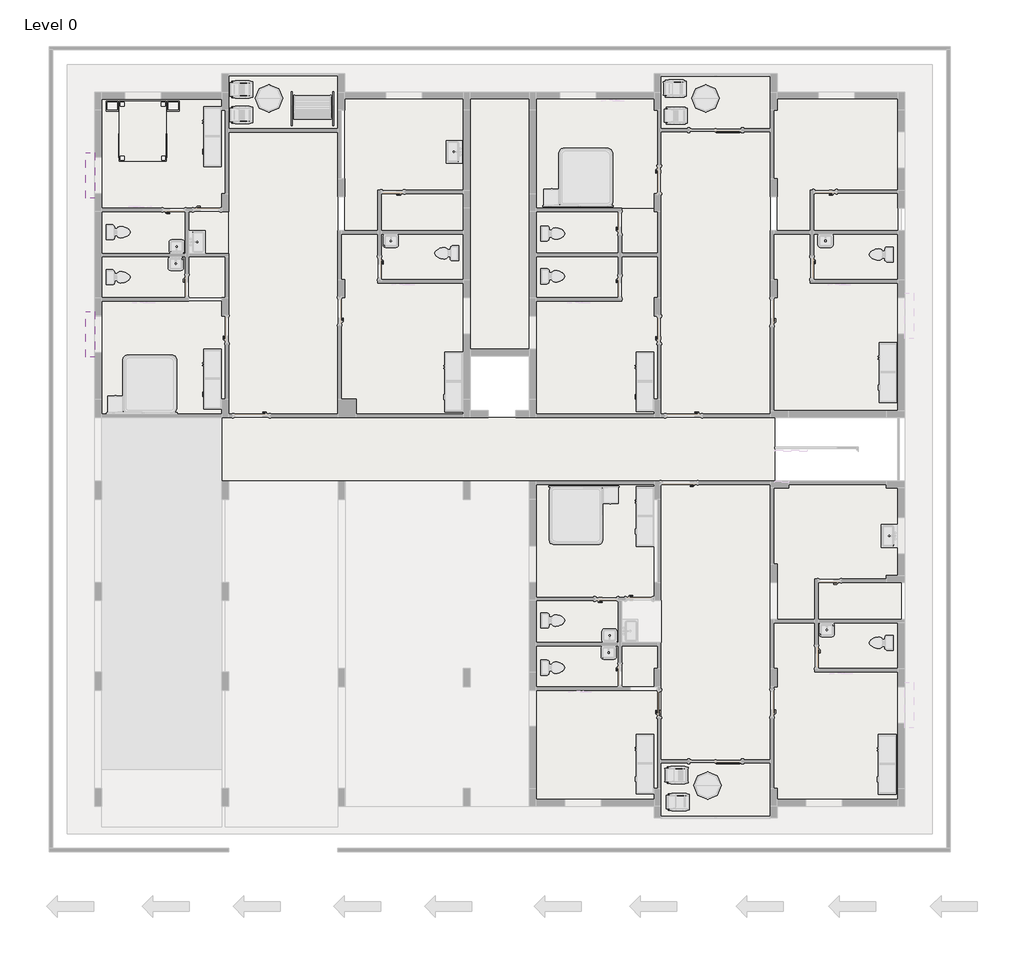
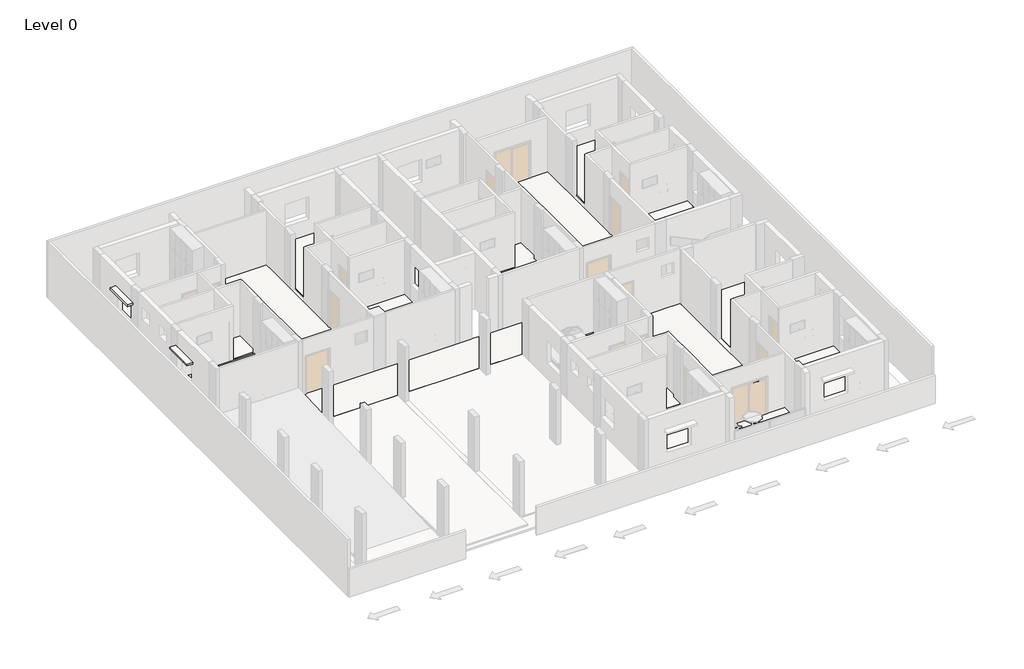
# One storey, part 4 of 6: 6 slabs.
"""IFC4 building model written with IfcOpenShell, lengths in millimetres."""

from ifc_helpers import new_model, si_unit, frame, origin, origin_with_axes, place, context, project, spatial, polyline, circle_curve, outline, extrude, element, save
from ifc_brep_helpers import plane_surface, cylinder_surface, revolved_surface, advanced_brep

model = new_model("IFC4")

# Units and contexts
model_context = context("Model", 3, world=origin())
ifc_project = project(units=[si_unit("LENGTHUNIT", "METRE", prefix="MILLI")], contexts=[model_context])

# Site, building, storey
site = spatial("IfcSite", under=ifc_project)
building = spatial("IfcBuilding", under=site)
storey = spatial("IfcBuildingStorey", under=building, Name="Level 0", Elevation=0.0)

# Slabs
placement = place(None, origin())
element("IfcSlab", 1, at=placement, inside=storey, context=model_context, shape_type="SweptSolid", body=[
    extrude(outline(polyline([(4028.5598466, -6653.8517861), (4028.5598466, -8050.8607795), (1285.3598461, -8050.8607795), (1285.3598461, -6653.8517861), (4028.5598466, -6653.8517861)])), frame((0.0, 0.0, -50.8), z_axis=(0.0, 0.0, 1.0), x_axis=(1.0, 0.0, 0.0)), (0.0, 0.0, 1.0), 50.8),
    extrude(outline(polyline([(4028.5598461, -8165.1517861), (4028.5598461, -9536.8048446), (1285.3598461, -9536.8048446), (1285.3598461, -8165.1517861), (4028.5598461, -8165.1517861)])), frame((0.0, 0.0, -50.8), z_axis=(0.0, 0.0, 1.0), x_axis=(1.0, 0.0, 0.0)), (0.0, 0.0, 1.0), 50.8),
    extrude(outline(polyline([(5343.0098461, -9536.7517862), (4142.8598461, -9536.7517862), (4142.8598461, -8165.1517861), (5343.0098461, -8165.1517861), (5343.0098461, -9536.7517862)])), frame((0.0, 0.0, -50.8), z_axis=(0.0, 0.0, 1.0), x_axis=(1.0, 0.0, 0.0)), (0.0, 0.0, 1.0), 50.8),
    extrude(outline(polyline([(10715.0567876, -7288.8517861), (10715.0567876, -6044.2517861), (13496.409846, -6044.2517861), (13496.409846, -7288.8517861), (10715.0567876, -7288.8517861)])), frame((0.0, 0.0, -50.8), z_axis=(0.0, 0.0, 1.0), x_axis=(1.0, 0.0, 0.0)), (0.0, 0.0, 1.0), 50.8),
    extrude(outline(polyline([(-5344.0401539, 10921.8022446), (-5344.0401539, 9143.8022446), (-9001.6401539, 9143.8022446), (-9001.6401539, 10921.8022446), (-5344.0401539, 10921.8022446)])), frame((0.0, 0.0, -50.8), z_axis=(0.0, 0.0, 1.0), x_axis=(1.0, 0.0, 0.0)), (0.0, 0.0, 1.0), 50.8),
    extrude(outline(polyline([(5462.3098461, -9651.0517861), (5462.3098461, -10565.4518735), (5343.0098461, -10565.4518735), (5343.0098461, -12927.6517861), (5228.6965978, -12927.6517861), (5228.6965978, -13308.6517861), (1285.3598461, -13308.6517861), (1285.3598461, -9651.0517861), (5462.3098461, -9651.0517861)])), frame((0.0, 0.0, -50.8), z_axis=(0.0, 0.0, 1.0), x_axis=(1.0, 0.0, 0.0)), (0.0, 0.0, 1.0), 50.8),
    extrude(outline(polyline([(5462.3098461, -6653.8517861), (5462.3098461, -8050.8607795), (4142.8598461, -8050.8607795), (4142.8598461, -6653.8517861), (5462.3098461, -6653.8517861)])), frame((0.0, 0.0, -50.8), z_axis=(0.0, 0.0, 1.0), x_axis=(1.0, 0.0, 0.0)), (0.0, 0.0, 1.0), 50.8),
    extrude(outline(polyline([(-9001.6401539, 6361.3562752), (-9001.6401539, 4965.5022446), (-10335.1401539, 4965.5022446), (-10335.1401539, 6361.3562752), (-9001.6401539, 6361.3562752)])), frame((0.0, 0.0, -50.8), z_axis=(0.0, 0.0, 1.0), x_axis=(1.0, 0.0, 0.0)), (0.0, 0.0, 1.0), 50.8),
])
element("IfcSlab", 2, ObjectType="4\"", at=placement, inside=storey, context=model_context, shape_type="SweptSolid", body=[
    extrude(outline(polyline([(-13783.1901539, 3022.4022446), (-13478.3901539, 3022.4022446), (-13478.3901539, 1498.4022446), (-13783.1901539, 1498.4022446), (-13783.1901539, 3022.4022446)])), frame((0.0, 0.0, 2108.2), z_axis=(0.0, 0.0, 1.0), x_axis=(1.0, 0.0, 0.0)), (0.0, 0.0, 1.0), 101.6),
])
element("IfcSlab", 3, ObjectType="4\"", at=placement, inside=storey, context=model_context, shape_type="SweptSolid", body=[
    extrude(outline(polyline([(-13783.190154, 8342.5562752), (-13478.3901539, 8342.5562752), (-13478.3901539, 6818.5562752), (-13783.190154, 6818.5562752), (-13783.190154, 8342.5562752)])), frame((0.0, 0.0, 2108.2), z_axis=(0.0, 0.0, 1.0), x_axis=(1.0, 0.0, 0.0)), (0.0, 0.0, 1.0), 101.6),
])
element("IfcSlab", 4, ObjectType="Tile", at=placement, inside=storey, context=model_context, shape_type="AdvancedBrep", body=[
    advanced_brep(
    [(-9230.2401539, 10133.2562752, 0.0), (-9230.2401539, 9752.2562752, 0.0), (-9115.9401539, 9752.2562752, 0.0), (-9115.9401539, 6972.1022446, 0.0), (-9230.2401539, 6972.1022446, 0.0), (-9230.2401539, 6476.8022446, 0.0), (-13249.7901539, 6476.8022446, 0.0), (-13249.7901539, 10133.2562752, 0.0), (-12669.0887417, 8172.6340818, 0.0), (-12666.8305798, 8172.6340818, 0.0), (-12666.8305798, 8969.1064638, 0.0), (-12669.0887417, 8969.1064638, 0.0), (-12689.9697227, 10058.1316218, 0.0), (-13099.9697227, 10058.1316218, 0.0), (-13099.9697227, 9728.1316218, 0.0), (-12689.9697227, 9728.1316218, 0.0), (-10645.1697227, 10058.1316218, 0.0), (-11055.1697227, 10058.1316218, 0.0), (-11055.1697227, 9728.1316218, 0.0), (-10645.1697227, 9728.1316218, 0.0), (-12459.9697227, 8051.5316218, 0.0), (-12459.9697227, 8251.5316218, 0.0), (-12659.9697227, 8251.5316218, 0.0), (-12659.9697227, 8051.5316218, 0.0), (-11285.1697227, 8051.5316218, 0.0), (-11085.1697227, 8051.5316218, 0.0), (-11085.1697227, 8251.5316218, 0.0), (-11285.1697227, 8251.5316218, 0.0), (-11285.1697227, 10058.1316218, 0.0), (-11285.1697227, 9858.1316218, 0.0), (-11085.1697227, 9858.1316218, 0.0), (-11085.1697227, 10058.1316218, 0.0), (-12459.9697227, 10058.1316218, 0.0), (-12659.9697227, 10058.1316218, 0.0), (-12659.9697227, 9858.1316218, 0.0), (-12459.9697227, 9858.1316218, 0.0), (-9230.2401539, 9752.2562752, 76.2), (-9230.2401539, 10133.2562752, 76.2), (-13249.7901539, 10133.2562752, 76.2), (-13249.7901539, 6476.8022446, 76.2), (-9230.2401539, 6476.8022446, 76.2), (-9230.2401539, 6972.1022446, 76.2), (-9115.9401539, 6972.1022446, 76.2), (-9115.9401539, 9752.2562752, 76.2), (-12659.9697227, 10058.1316218, 76.2), (-11085.1697227, 10058.1316218, 76.2), (-11085.1697227, 8051.5316218, 76.2), (-12659.9697227, 8051.5316218, 76.2), (-10645.1697227, 9728.1316218, 76.2), (-11055.1697227, 9728.1316218, 76.2), (-11055.1697227, 10058.1316218, 76.2), (-10645.1697227, 10058.1316218, 76.2), (-12689.9697227, 9728.1316218, 76.2), (-13099.9697227, 9728.1316218, 76.2), (-13099.9697227, 10058.1316218, 76.2), (-12689.9697227, 10058.1316218, 76.2), (-12668.2662368, 8172.6340818, 76.2), (-12669.2815845, 8172.6340818, 76.2), (-12669.2815845, 8969.1064638, 76.2), (-12668.2662368, 8969.1064638, 76.2), (-11068.8512642, 8172.6340818, 76.2), (-11069.8590146, 8172.6340818, 76.2), (-11069.8590146, 8969.1064638, 76.2), (-11068.8512642, 8969.1064638, 76.2), (-11085.1697227, 8051.5316218, 60.0), (-11085.1697227, 10058.1316218, 60.0), (-12659.9697227, 10058.1316218, 60.0), (-12659.9697227, 8051.5316218, 60.0), (-12619.9697227, 10018.1316218, 60.0), (-12499.9697227, 10018.1316218, 60.0), (-12499.9697227, 9898.1316218, 60.0), (-12619.9697227, 9898.1316218, 60.0), (-11249.1033441, 10018.1316218, 60.0), (-11125.1697227, 10018.1316218, 60.0), (-11125.1697227, 9898.1316218, 60.0), (-11249.1033441, 9898.1316218, 60.0), (-12619.9697227, 8211.5316218, 60.0), (-12499.9697227, 8211.5316218, 60.0), (-12499.9697227, 8091.5316218, 60.0), (-12619.9697227, 8091.5316218, 60.0), (-11245.1697227, 8211.5316218, 60.0), (-11125.1697227, 8211.5316218, 60.0), (-11125.1697227, 8091.5316218, 60.0), (-11245.1697227, 8091.5316218, 60.0), (-10685.1697227, 10018.1316218, 50.0), (-10685.1697227, 10018.1316218, 60.0), (-11015.1697227, 10018.1316218, 60.0), (-11015.1697227, 10018.1316218, 50.0), (-11015.1697227, 9768.1316218, 60.0), (-11015.1697227, 9768.1316218, 50.0), (-10685.1697227, 9768.1316218, 60.0), (-10685.1697227, 9768.1316218, 50.0), (-12729.9697227, 10018.1316218, 50.0), (-12729.9697227, 10018.1316218, 60.0), (-13059.9697227, 10018.1316218, 60.0), (-13059.9697227, 10018.1316218, 50.0), (-13059.9697227, 9768.1316218, 60.0), (-13059.9697227, 9768.1316218, 50.0), (-12729.9697227, 9768.1316218, 60.0), (-12729.9697227, 9768.1316218, 50.0), (-11055.1697227, 10058.1316218, 60.0), (-11055.1697227, 9728.1316218, 60.0), (-10645.1697227, 9728.1316218, 60.0), (-10645.1697227, 10058.1316218, 60.0), (-13099.9697227, 10058.1316218, 60.0), (-13099.9697227, 9728.1316218, 60.0), (-12689.9697227, 9728.1316218, 60.0), (-12689.9697227, 10058.1316218, 60.0), (-12499.9697227, 10018.1316218, 50.0), (-12619.9697227, 10018.1316218, 50.0), (-12619.9697227, 9898.1316218, 50.0), (-12499.9697227, 9898.1316218, 50.0), (-11125.1697227, 10018.1316218, 50.0), (-11249.1033441, 10018.1316218, 50.0), (-11249.1033441, 9898.1316218, 50.0), (-11125.1697227, 9898.1316218, 50.0), (-12499.9697227, 8211.5316218, 50.0), (-12619.9697227, 8211.5316218, 50.0), (-12619.9697227, 8091.5316218, 50.0), (-12499.9697227, 8091.5316218, 50.0), (-11125.1697227, 8211.5316218, 50.0), (-11245.1697227, 8211.5316218, 50.0), (-11245.1697227, 8091.5316218, 50.0), (-11125.1697227, 8091.5316218, 50.0), (-11065.9668196, 8172.6340818, 0.0), (-11080.438493, 8172.6340818, 25.8475978), (-11079.4802179, 8172.6340818, 25.5617504), (-11065.1424088, 8172.6340818, 0.8244107), (-12680.5715859, 8172.6340818, 27.6877586), (-12679.6113712, 8172.6340818, 27.4084957), (-12679.6113712, 8969.1064638, 27.4084957), (-12680.5715859, 8969.1064638, 27.6877586), (-11065.1424088, 8969.1064638, 0.8244107), (-11079.4802179, 8969.1064638, 25.5617504), (-11080.438493, 8969.1064638, 25.8475978), (-11065.9668196, 8969.1064638, 0.0), (-13099.9697227, 10058.1316218, 50.0), (-12689.9697227, 10058.1316218, 50.0), (-12689.9697227, 9728.1316218, 50.0), (-13099.9697227, 9728.1316218, 50.0), (-11055.1697227, 10058.1316218, 50.0), (-10645.1697227, 10058.1316218, 50.0), (-10645.1697227, 9728.1316218, 50.0), (-11055.1697227, 9728.1316218, 50.0), (-12459.9697227, 8251.5316218, 50.0), (-12459.9697227, 8051.5316218, 50.0), (-12659.9697227, 8051.5316218, 50.0), (-12659.9697227, 8251.5316218, 50.0), (-11085.1697227, 8051.5316218, 50.0), (-11285.1697227, 8051.5316218, 50.0), (-11285.1697227, 8251.5316218, 50.0), (-11085.1697227, 8251.5316218, 50.0), (-11285.1697227, 9858.1316218, 50.0), (-11285.1697227, 10058.1316218, 50.0), (-11085.1697227, 10058.1316218, 50.0), (-11085.1697227, 9858.1316218, 50.0), (-12659.9697227, 10058.1316218, 50.0), (-12459.9697227, 10058.1316218, 50.0), (-12459.9697227, 9858.1316218, 50.0), (-12659.9697227, 9858.1316218, 50.0)],
    [
        (0, 1),
        (1, 2),
        (2, 3),
        (3, 4),
        (4, 5),
        (5, 6),
        (6, 7),
        (7, 0),
        (8, 9),
        (9, 10),
        (10, 11),
        (11, 8),
        (12, 13),
        (13, 14),
        (14, 15),
        (15, 12),
        (16, 17),
        (17, 18),
        (18, 19),
        (19, 16),
        (20, 21),
        (21, 22),
        (22, 23),
        (23, 20),
        (24, 25),
        (25, 26),
        (26, 27),
        (27, 24),
        (28, 29),
        (29, 30),
        (30, 31),
        (31, 28),
        (32, 33),
        (33, 34),
        (34, 35),
        (35, 32),
        (36, 37),
        (37, 38),
        (38, 39),
        (39, 40),
        (40, 41),
        (41, 42),
        (42, 43),
        (43, 36),
        (44, 45),
        (45, 46),
        (46, 47),
        (47, 44),
        (48, 49),
        (49, 50),
        (50, 51),
        (51, 48),
        (52, 53),
        (53, 54),
        (54, 55),
        (55, 52),
        (56, 57),
        (57, 58),
        (58, 59),
        (59, 56),
        (60, 61),
        (61, 62),
        (62, 63),
        (63, 60),
        (0, 37),
        (36, 1),
        (43, 2),
        (42, 3),
        (41, 4),
        (40, 5),
        (39, 6),
        (38, 7),
        (64, 65),
        (65, 66),
        (66, 67),
        (67, 64),
        (68, 69),
        (69, 70),
        (70, 71),
        (71, 68),
        (72, 73),
        (73, 74),
        (74, 75),
        (75, 72),
        (76, 77),
        (77, 78),
        (78, 79),
        (79, 76),
        (80, 81),
        (81, 82),
        (82, 83),
        (83, 80),
        (65, 45),
        (44, 66),
        (47, 67),
        (46, 64),
        (84, 85),
        (85, 86),
        (86, 87),
        (87, 84),
        (86, 88),
        (88, 89),
        (89, 87),
        (88, 90),
        (90, 91),
        (91, 89),
        (84, 91),
        (90, 85),
        (92, 93),
        (93, 94),
        (94, 95),
        (95, 92),
        (94, 96),
        (96, 97),
        (97, 95),
        (96, 98),
        (98, 99),
        (99, 97),
        (92, 99),
        (98, 93),
        (100, 101),
        (101, 102),
        (102, 103),
        (103, 100),
        (104, 105),
        (105, 106),
        (106, 107),
        (107, 104),
        (101, 49),
        (48, 102),
        (51, 103),
        (50, 100),
        (105, 53),
        (52, 106),
        (55, 107),
        (54, 104),
        (108, 69),
        (68, 109),
        (109, 108),
        (71, 110),
        (110, 109),
        (70, 111),
        (111, 110),
        (108, 111),
        (112, 73),
        (72, 113),
        (113, 112),
        (75, 114),
        (114, 113),
        (74, 115),
        (115, 114),
        (112, 115),
        (116, 77),
        (76, 117),
        (117, 116),
        (79, 118),
        (118, 117),
        (78, 119),
        (119, 118),
        (116, 119),
        (120, 81),
        (80, 121),
        (121, 120),
        (83, 122),
        (122, 121),
        (82, 123),
        (123, 122),
        (120, 123),
        (124, 125, circle_curve(frame((-11060.6581831, 8172.6340818, 19.947257), z_axis=(0.0, 1.0, 0.0), x_axis=(1.0, 0.0, 0.0)), 20.6415766)),
        (125, 61, circle_curve(frame((-11378.5350117, 8172.6340818, 114.7678954), z_axis=(0.0, -1.0, 0.0), x_axis=(1.0, 0.0, 0.0)), 311.0761221)),
        (60, 126, circle_curve(frame((-11378.5350117, 8172.6340818, 114.7678954), z_axis=(0.0, 1.0, 0.0), x_axis=(1.0, 0.0, 0.0)), 312.0761221)),
        (126, 127, circle_curve(frame((-11060.6581831, 8172.6340818, 19.947257), z_axis=(0.0, -1.0, 0.0), x_axis=(1.0, 0.0, 0.0)), 19.6415766)),
        (127, 124),
        (8, 128, circle_curve(frame((-12657.5756771, 8172.6340818, 20.9997703), z_axis=(0.0, 1.0, 0.0), x_axis=(1.0, 0.0, 0.0)), 23.9487162)),
        (128, 57, circle_curve(frame((-13120.6038463, 8172.6340818, 155.6640283), z_axis=(0.0, -1.0, 0.0), x_axis=(1.0, 0.0, 0.0)), 458.2644606)),
        (56, 129, circle_curve(frame((-13120.6038463, 8172.6340818, 155.6640283), z_axis=(0.0, 1.0, 0.0), x_axis=(1.0, 0.0, 0.0)), 459.2644606)),
        (129, 9, circle_curve(frame((-12657.5756771, 8172.6340818, 20.9997703), z_axis=(0.0, -1.0, 0.0), x_axis=(1.0, 0.0, 0.0)), 22.9487162)),
        (10, 130, circle_curve(frame((-12657.5756771, 8969.1064638, 20.9997703), z_axis=(0.0, 1.0, 0.0), x_axis=(1.0, 0.0, 0.0)), 22.9487162)),
        (130, 59, circle_curve(frame((-13120.6038463, 8969.1064638, 155.6640283), z_axis=(0.0, -1.0, 0.0), x_axis=(1.0, 0.0, 0.0)), 459.2644606)),
        (58, 131, circle_curve(frame((-13120.6038463, 8969.1064638, 155.6640283), z_axis=(0.0, 1.0, 0.0), x_axis=(1.0, 0.0, 0.0)), 458.2644606)),
        (131, 11, circle_curve(frame((-12657.5756771, 8969.1064638, 20.9997703), z_axis=(0.0, -1.0, 0.0), x_axis=(1.0, 0.0, 0.0)), 23.9487162)),
        (132, 133, circle_curve(frame((-11060.6581831, 8969.1064638, 19.947257), z_axis=(0.0, 1.0, 0.0), x_axis=(1.0, 0.0, 0.0)), 19.6415766)),
        (133, 63, circle_curve(frame((-11378.5350117, 8969.1064638, 114.7678954), z_axis=(0.0, -1.0, 0.0), x_axis=(1.0, 0.0, 0.0)), 312.0761221)),
        (62, 134, circle_curve(frame((-11378.5350117, 8969.1064638, 114.7678954), z_axis=(0.0, 1.0, 0.0), x_axis=(1.0, 0.0, 0.0)), 311.0761221)),
        (134, 135, circle_curve(frame((-11060.6581831, 8969.1064638, 19.947257), z_axis=(0.0, -1.0, 0.0), x_axis=(1.0, 0.0, 0.0)), 20.6415766)),
        (135, 132),
        (125, 134),
        (133, 126),
        (128, 131),
        (130, 129),
        (136, 137),
        (137, 138),
        (138, 139),
        (139, 136),
        (140, 141),
        (141, 142),
        (142, 143),
        (143, 140),
        (136, 13),
        (12, 137),
        (139, 14),
        (138, 15),
        (140, 17),
        (16, 141),
        (143, 18),
        (142, 19),
        (144, 145),
        (145, 146),
        (146, 147),
        (147, 144),
        (148, 149),
        (149, 150),
        (150, 151),
        (151, 148),
        (152, 153),
        (153, 154),
        (154, 155),
        (155, 152),
        (156, 157),
        (157, 158),
        (158, 159),
        (159, 156),
        (144, 21),
        (20, 145),
        (147, 22),
        (146, 23),
        (148, 25),
        (24, 149),
        (151, 26),
        (150, 27),
        (152, 29),
        (28, 153),
        (155, 30),
        (154, 31),
        (156, 33),
        (32, 157),
        (159, 34),
        (158, 35),
        (124, 135),
        (127, 132),
    ],
    [
        plane_surface(frame((-9230.2401539, 10361.8562752, 0.0), z_axis=(0.0, 0.0, -1.0), x_axis=(0.0, -1.0, 0.0))),
        plane_surface(frame((-9230.2401539, 10361.8562752, 76.2), z_axis=(0.0, 0.0, 1.0), x_axis=(0.0, 1.0, 0.0))),
        plane_surface(frame((-9230.2401539, 10133.2562752, 0.0), z_axis=(1.0, 0.0, 0.0), x_axis=(0.0, 0.0, 1.0))),
        plane_surface(frame((-9230.2401539, 9752.2562752, 0.0), z_axis=(0.0, 1.0, 0.0), x_axis=(0.0, 0.0, 1.0))),
        plane_surface(frame((-9115.9401539, 9752.2562752, 0.0), z_axis=(1.0, 0.0, 0.0), x_axis=(0.0, 0.0, 1.0))),
        plane_surface(frame((-9115.9401539, 6972.1022446, 0.0), z_axis=(0.0, -1.0, 0.0), x_axis=(0.0, 0.0, 1.0))),
        plane_surface(frame((-9230.2401539, 6972.1022446, 0.0), z_axis=(1.0, 0.0, 0.0), x_axis=(0.0, 0.0, 1.0))),
        plane_surface(frame((-9230.2401539, 6476.8022446, 0.0), z_axis=(0.0, -1.0, 0.0), x_axis=(0.0, 0.0, 1.0))),
        plane_surface(frame((-13249.7901539, 6476.8022446, 0.0), z_axis=(-1.0, 0.0, 0.0), x_axis=(0.0, 0.0, 1.0))),
        plane_surface(frame((-13249.7901539, 10133.2562752, 0.0), z_axis=(0.0, 1.0, 0.0), x_axis=(0.0, 0.0, 1.0))),
        plane_surface(frame((-12659.9697227, 10058.1316218, 60.0), z_axis=(0.0, 0.0, 1.0), x_axis=(1.0, 0.0, 0.0))),
        plane_surface(frame((-11085.1697227, 10058.1316218, 286.5360466), z_axis=(0.0, -1.0, 0.0), x_axis=(0.0, 0.0, -1.0))),
        plane_surface(frame((-12659.9697227, 10058.1316218, 286.5360466), z_axis=(1.0, 0.0, 0.0), x_axis=(0.0, 0.0, -1.0))),
        plane_surface(frame((-12659.9697227, 8051.5316218, 286.5360466), z_axis=(0.0, 1.0, 0.0), x_axis=(0.0, 0.0, -1.0))),
        plane_surface(frame((-11085.1697227, 8051.5316218, 286.5360466), z_axis=(-1.0, 0.0, 0.0), x_axis=(0.0, 0.0, -1.0))),
        plane_surface(frame((-10685.1697227, 10018.1316218, 60.0), z_axis=(0.0, -1.0, 0.0), x_axis=(0.0, 0.0, -1.0))),
        plane_surface(frame((-11015.1697227, 10018.1316218, 60.0), z_axis=(1.0, 0.0, 0.0), x_axis=(0.0, 0.0, -1.0))),
        plane_surface(frame((-11015.1697227, 9768.1316218, 60.0), z_axis=(0.0, 1.0, 0.0), x_axis=(0.0, 0.0, -1.0))),
        plane_surface(frame((-10685.1697227, 9768.1316218, 60.0), z_axis=(-1.0, 0.0, 0.0), x_axis=(0.0, 0.0, -1.0))),
        plane_surface(frame((-12729.9697227, 10018.1316218, 60.0), z_axis=(0.0, -1.0, 0.0), x_axis=(0.0, 0.0, -1.0))),
        plane_surface(frame((-13059.9697227, 10018.1316218, 60.0), z_axis=(1.0, 0.0, 0.0), x_axis=(0.0, 0.0, -1.0))),
        plane_surface(frame((-13059.9697227, 9768.1316218, 60.0), z_axis=(0.0, 1.0, 0.0), x_axis=(0.0, 0.0, -1.0))),
        plane_surface(frame((-12729.9697227, 9768.1316218, 60.0), z_axis=(-1.0, 0.0, 0.0), x_axis=(0.0, 0.0, -1.0))),
        plane_surface(frame((-10645.1697227, 9728.1316218, 60.0), z_axis=(0.0, 0.0, 1.0), x_axis=(-1.0, 0.0, 0.0))),
        plane_surface(frame((-11055.1697227, 9728.1316218, 350.5398437), z_axis=(0.0, 1.0, 0.0), x_axis=(0.0, 0.0, -1.0))),
        plane_surface(frame((-10645.1697227, 9728.1316218, 350.5398437), z_axis=(-1.0, 0.0, 0.0), x_axis=(0.0, 0.0, -1.0))),
        plane_surface(frame((-10645.1697227, 10058.1316218, 350.5398437), z_axis=(0.0, -1.0, 0.0), x_axis=(0.0, 0.0, -1.0))),
        plane_surface(frame((-11055.1697227, 10058.1316218, 350.5398437), z_axis=(1.0, 0.0, 0.0), x_axis=(0.0, 0.0, -1.0))),
        plane_surface(frame((-13099.9697227, 9728.1316218, 350.5398437), z_axis=(0.0, 1.0, 0.0), x_axis=(0.0, 0.0, -1.0))),
        plane_surface(frame((-12689.9697227, 9728.1316218, 350.5398437), z_axis=(-1.0, 0.0, 0.0), x_axis=(0.0, 0.0, -1.0))),
        plane_surface(frame((-12689.9697227, 10058.1316218, 350.5398437), z_axis=(0.0, -1.0, 0.0), x_axis=(0.0, 0.0, -1.0))),
        plane_surface(frame((-13099.9697227, 10058.1316218, 350.5398437), z_axis=(1.0, 0.0, 0.0), x_axis=(0.0, 0.0, -1.0))),
        plane_surface(frame((-12499.9697227, 10018.1316218, 67.4567817), z_axis=(0.0, -1.0, 0.0), x_axis=(0.0, 0.0, -1.0))),
        plane_surface(frame((-12619.9697227, 10018.1316218, 67.4567817), z_axis=(1.0, 0.0, 0.0), x_axis=(0.0, 0.0, -1.0))),
        plane_surface(frame((-12619.9697227, 9898.1316218, 67.4567817), z_axis=(0.0, 1.0, 0.0), x_axis=(0.0, 0.0, -1.0))),
        plane_surface(frame((-12499.9697227, 9898.1316218, 67.4567817), z_axis=(-1.0, 0.0, 0.0), x_axis=(0.0, 0.0, -1.0))),
        plane_surface(frame((-11125.1697227, 10018.1316218, 67.4567817), z_axis=(0.0, -1.0, 0.0), x_axis=(0.0, 0.0, -1.0))),
        plane_surface(frame((-11249.1033441, 10018.1316218, 67.4567817), z_axis=(1.0, 0.0, 0.0), x_axis=(0.0, 0.0, -1.0))),
        plane_surface(frame((-11249.1033441, 9898.1316218, 67.4567817), z_axis=(0.0, 1.0, 0.0), x_axis=(0.0, 0.0, -1.0))),
        plane_surface(frame((-11125.1697227, 9898.1316218, 67.4567817), z_axis=(-1.0, 0.0, 0.0), x_axis=(0.0, 0.0, -1.0))),
        plane_surface(frame((-12499.9697227, 8211.5316218, 67.4567817), z_axis=(0.0, -1.0, 0.0), x_axis=(0.0, 0.0, -1.0))),
        plane_surface(frame((-12619.9697227, 8211.5316218, 67.4567817), z_axis=(1.0, 0.0, 0.0), x_axis=(0.0, 0.0, -1.0))),
        plane_surface(frame((-12619.9697227, 8091.5316218, 67.4567817), z_axis=(0.0, 1.0, 0.0), x_axis=(0.0, 0.0, -1.0))),
        plane_surface(frame((-12499.9697227, 8091.5316218, 67.4567817), z_axis=(-1.0, 0.0, 0.0), x_axis=(0.0, 0.0, -1.0))),
        plane_surface(frame((-11125.1697227, 8211.5316218, 67.4567817), z_axis=(0.0, -1.0, 0.0), x_axis=(0.0, 0.0, -1.0))),
        plane_surface(frame((-11245.1697227, 8211.5316218, 67.4567817), z_axis=(1.0, 0.0, 0.0), x_axis=(0.0, 0.0, -1.0))),
        plane_surface(frame((-11245.1697227, 8091.5316218, 67.4567817), z_axis=(0.0, 1.0, 0.0), x_axis=(0.0, 0.0, -1.0))),
        plane_surface(frame((-11125.1697227, 8091.5316218, 67.4567817), z_axis=(-1.0, 0.0, 0.0), x_axis=(0.0, 0.0, -1.0))),
        plane_surface(frame((-11140.0703301, 8172.6340818, 452.0728643), z_axis=(0.0, 1.0, 0.0), x_axis=(0.0, 0.0, -1.0))),
        plane_surface(frame((-11140.0703301, 8969.1064638, 452.0728643), z_axis=(0.0, -1.0, 0.0), x_axis=(0.0, 0.0, 1.0))),
        cylinder_surface(frame((-11378.5350117, 8969.1064638, 114.7678954), z_axis=(0.0, 1.0, 0.0), x_axis=(1.0, 0.0, 0.0)), 311.0761221),
        revolved_surface(polyline([(-11066.4588896, 8172.6340818, 114.7678954), (-11066.4588896, 8969.1064638, 114.7678954)]), (-11378.5350117, 8969.1064638, 114.7678954), (0.0, -1.0, 0.0)),
        cylinder_surface(frame((-13120.6038463, 8969.1064638, 155.6640283), z_axis=(0.0, 1.0, 0.0), x_axis=(1.0, 0.0, 0.0)), 458.2644606),
        revolved_surface(polyline([(-12661.339385700001, 8172.6340818, 155.6640283), (-12661.339385700001, 8969.1064638, 155.6640283)]), (-13120.6038463, 8969.1064638, 155.6640283), (0.0, -1.0, 0.0)),
        plane_surface(frame((-13205.861526, 10058.1316218, 50.0), z_axis=(0.0, 0.0, -1.0), x_axis=(-1.0, 0.0, 0.0))),
        plane_surface(frame((-12689.9697227, 10058.1316218, 50.0), z_axis=(0.0, -1.0, 0.0), x_axis=(0.0, 0.0, -1.0))),
        plane_surface(frame((-13099.9697227, 10058.1316218, 50.0), z_axis=(1.0, 0.0, 0.0), x_axis=(0.0, 0.0, -1.0))),
        plane_surface(frame((-13099.9697227, 9728.1316218, 50.0), z_axis=(0.0, 1.0, 0.0), x_axis=(0.0, 0.0, -1.0))),
        plane_surface(frame((-12689.9697227, 9728.1316218, 50.0), z_axis=(-1.0, 0.0, 0.0), x_axis=(0.0, 0.0, -1.0))),
        plane_surface(frame((-10645.1697227, 10058.1316218, 50.0), z_axis=(0.0, -1.0, 0.0), x_axis=(0.0, 0.0, -1.0))),
        plane_surface(frame((-11055.1697227, 10058.1316218, 50.0), z_axis=(1.0, 0.0, 0.0), x_axis=(0.0, 0.0, -1.0))),
        plane_surface(frame((-11055.1697227, 9728.1316218, 50.0), z_axis=(0.0, 1.0, 0.0), x_axis=(0.0, 0.0, -1.0))),
        plane_surface(frame((-10645.1697227, 9728.1316218, 50.0), z_axis=(-1.0, 0.0, 0.0), x_axis=(0.0, 0.0, -1.0))),
        plane_surface(frame((-12459.9697227, 8061.1968197, 50.0), z_axis=(0.0, 0.0, -1.0), x_axis=(0.0, 1.0, 0.0))),
        plane_surface(frame((-12459.9697227, 8051.5316218, 50.0), z_axis=(-1.0, 0.0, 0.0), x_axis=(0.0, 0.0, -1.0))),
        plane_surface(frame((-12459.9697227, 8251.5316218, 50.0), z_axis=(0.0, -1.0, 0.0), x_axis=(0.0, 0.0, -1.0))),
        plane_surface(frame((-12659.9697227, 8251.5316218, 50.0), z_axis=(1.0, 0.0, 0.0), x_axis=(0.0, 0.0, -1.0))),
        plane_surface(frame((-12659.9697227, 8051.5316218, 50.0), z_axis=(0.0, 1.0, 0.0), x_axis=(0.0, 0.0, -1.0))),
        plane_surface(frame((-11285.1697227, 8051.5316218, 50.0), z_axis=(0.0, 1.0, 0.0), x_axis=(0.0, 0.0, -1.0))),
        plane_surface(frame((-11085.1697227, 8051.5316218, 50.0), z_axis=(-1.0, 0.0, 0.0), x_axis=(0.0, 0.0, -1.0))),
        plane_surface(frame((-11085.1697227, 8251.5316218, 50.0), z_axis=(0.0, -1.0, 0.0), x_axis=(0.0, 0.0, -1.0))),
        plane_surface(frame((-11285.1697227, 8251.5316218, 50.0), z_axis=(1.0, 0.0, 0.0), x_axis=(0.0, 0.0, -1.0))),
        plane_surface(frame((-11285.1697227, 10058.1316218, 50.0), z_axis=(1.0, 0.0, 0.0), x_axis=(0.0, 0.0, -1.0))),
        plane_surface(frame((-11285.1697227, 9858.1316218, 50.0), z_axis=(0.0, 1.0, 0.0), x_axis=(0.0, 0.0, -1.0))),
        plane_surface(frame((-11085.1697227, 9858.1316218, 50.0), z_axis=(-1.0, 0.0, 0.0), x_axis=(0.0, 0.0, -1.0))),
        plane_surface(frame((-11085.1697227, 10058.1316218, 50.0), z_axis=(0.0, -1.0, 0.0), x_axis=(0.0, 0.0, -1.0))),
        plane_surface(frame((-12459.9697227, 10058.1316218, 50.0), z_axis=(0.0, -1.0, 0.0), x_axis=(0.0, 0.0, -1.0))),
        plane_surface(frame((-12659.9697227, 10058.1316218, 50.0), z_axis=(1.0, 0.0, 0.0), x_axis=(0.0, 0.0, -1.0))),
        plane_surface(frame((-12659.9697227, 9858.1316218, 50.0), z_axis=(0.0, 1.0, 0.0), x_axis=(0.0, 0.0, -1.0))),
        plane_surface(frame((-12459.9697227, 9858.1316218, 50.0), z_axis=(-1.0, 0.0, 0.0), x_axis=(0.0, 0.0, -1.0))),
        revolved_surface(polyline([(-11040.016606500001, 8172.6340818, 19.947257), (-11040.016606500001, 8969.1064638, 19.947257)]), (-11060.6581831, 8969.1064638, 19.947257), (0.0, -1.0, 0.0)),
        plane_surface(frame((-11065.9668196, 8172.6340818, 0.0), z_axis=(-0.7071067811864398, 0.0, 0.7071067811866554), x_axis=(0.0, 1.0, 0.0))),
        cylinder_surface(frame((-11060.6581831, 8969.1064638, 19.947257), z_axis=(0.0, 1.0, 0.0), x_axis=(1.0, 0.0, 0.0)), 19.6415766),
        revolved_surface(polyline([(-12633.6269609, 8172.6340818, 20.9997703), (-12633.6269609, 8969.1064638, 20.9997703)]), (-12657.5756771, 8969.1064638, 20.9997703), (0.0, -1.0, 0.0)),
        cylinder_surface(frame((-12657.5756771, 8969.1064638, 20.9997703), z_axis=(0.0, 1.0, 0.0), x_axis=(1.0, 0.0, 0.0)), 22.9487162),
    ],
    [
        (0, [[1, 2, 3, 4, 5, 6, 7, 8], [9, 10, 11, 12], [13, 14, 15, 16], [17, 18, 19, 20], [21, 22, 23, 24], [25, 26, 27, 28], [29, 30, 31, 32], [33, 34, 35, 36]]),
        (1, [[37, 38, 39, 40, 41, 42, 43, 44], [45, 46, 47, 48], [49, 50, 51, 52], [53, 54, 55, 56], [57, 58, 59, 60], [61, 62, 63, 64]]),
        (2, [[-1, 65, -37, 66]]),
        (3, [[-2, -66, -44, 67]]),
        (4, [[-3, -67, -43, 68]]),
        (5, [[-4, -68, -42, 69]]),
        (6, [[-5, -69, -41, 70]]),
        (7, [[-6, -70, -40, 71]]),
        (8, [[-7, -71, -39, 72]]),
        (9, [[-8, -72, -38, -65]]),
        (10, [[73, 74, 75, 76], [77, 78, 79, 80], [81, 82, 83, 84], [85, 86, 87, 88], [89, 90, 91, 92]]),
        (11, [[-74, 93, -45, 94]]),
        (12, [[-75, -94, -48, 95]]),
        (13, [[-76, -95, -47, 96]]),
        (14, [[-73, -96, -46, -93]]),
        (15, [[97, 98, 99, 100]]),
        (16, [[-99, 101, 102, 103]]),
        (17, [[-102, 104, 105, 106]]),
        (18, [[-97, 107, -105, 108]]),
        (19, [[109, 110, 111, 112]]),
        (20, [[-111, 113, 114, 115]]),
        (21, [[-114, 116, 117, 118]]),
        (22, [[-109, 119, -117, 120]]),
        (23, [[121, 122, 123, 124], [-98, -108, -104, -101]]),
        (23, [[125, 126, 127, 128], [-110, -120, -116, -113]]),
        (24, [[-122, 129, -49, 130]]),
        (25, [[-123, -130, -52, 131]]),
        (26, [[-124, -131, -51, 132]]),
        (27, [[-121, -132, -50, -129]]),
        (28, [[-126, 133, -53, 134]]),
        (29, [[-127, -134, -56, 135]]),
        (30, [[-128, -135, -55, 136]]),
        (31, [[-125, -136, -54, -133]]),
        (32, [[137, -77, 138, 139]]),
        (33, [[-138, -80, 140, 141]]),
        (34, [[-140, -79, 142, 143]]),
        (35, [[-137, 144, -142, -78]]),
        (36, [[145, -81, 146, 147]]),
        (37, [[-146, -84, 148, 149]]),
        (38, [[-148, -83, 150, 151]]),
        (39, [[-145, 152, -150, -82]]),
        (40, [[153, -85, 154, 155]]),
        (41, [[-154, -88, 156, 157]]),
        (42, [[-156, -87, 158, 159]]),
        (43, [[-153, 160, -158, -86]]),
        (44, [[161, -89, 162, 163]]),
        (45, [[-162, -92, 164, 165]]),
        (46, [[-164, -91, 166, 167]]),
        (47, [[-161, 168, -166, -90]]),
        (48, [[169, 170, -61, 171, 172, 173]]),
        (48, [[174, 175, -57, 176, 177, -9]]),
        (49, [[178, 179, -59, 180, 181, -11]]),
        (49, [[182, 183, -63, 184, 185, 186]]),
        (50, [[187, -184, -62, -170]]),
        (51, [[188, -171, -64, -183]]),
        (52, [[189, -180, -58, -175]]),
        (53, [[190, -176, -60, -179]]),
        (54, [[191, 192, 193, 194], [-112, -115, -118, -119]]),
        (54, [[195, 196, 197, 198], [-100, -103, -106, -107]]),
        (55, [[-191, 199, -13, 200]]),
        (56, [[-194, 201, -14, -199]]),
        (57, [[-193, 202, -15, -201]]),
        (58, [[-192, -200, -16, -202]]),
        (59, [[-195, 203, -17, 204]]),
        (60, [[-198, 205, -18, -203]]),
        (61, [[-197, 206, -19, -205]]),
        (62, [[-196, -204, -20, -206]]),
        (63, [[207, 208, 209, 210], [-155, -157, -159, -160]]),
        (63, [[211, 212, 213, 214], [-163, -165, -167, -168]]),
        (63, [[215, 216, 217, 218], [-147, -149, -151, -152]]),
        (63, [[219, 220, 221, 222], [-139, -141, -143, -144]]),
        (64, [[-207, 223, -21, 224]]),
        (65, [[-210, 225, -22, -223]]),
        (66, [[-209, 226, -23, -225]]),
        (67, [[-208, -224, -24, -226]]),
        (68, [[-211, 227, -25, 228]]),
        (69, [[-214, 229, -26, -227]]),
        (70, [[-213, 230, -27, -229]]),
        (71, [[-212, -228, -28, -230]]),
        (72, [[-215, 231, -29, 232]]),
        (73, [[-218, 233, -30, -231]]),
        (74, [[-217, 234, -31, -233]]),
        (75, [[-216, -232, -32, -234]]),
        (76, [[-219, 235, -33, 236]]),
        (77, [[-222, 237, -34, -235]]),
        (78, [[-221, 238, -35, -237]]),
        (79, [[-220, -236, -36, -238]]),
        (80, [[-169, 239, -185, -187]]),
        (81, [[-173, 240, -186, -239]]),
        (82, [[-172, -188, -182, -240]]),
        (83, [[-174, -12, -181, -189]]),
        (84, [[-177, -190, -178, -10]]),
    ],
),
])
element("IfcSlab", 5, ObjectType="Tile", at=placement, inside=storey, context=model_context, shape_type="SweptSolid", body=[
    extrude(outline(polyline([(-5344.0401539, 9029.5022446), (-5344.0401539, -406.5977554), (-9001.6401539, -406.5977554), (-9001.6401539, 9029.5022446), (-5344.0401539, 9029.5022446)])), origin_with_axes(), (0.0, 0.0, 1.0), 76.2),
    extrude(outline(polyline([(-9230.2401539, 3365.3022446), (-9230.2401539, 2871.1482139), (-9115.9401539, 2871.1482139), (-9115.9401539, 89.8788513), (-9230.2401539, 89.8788513), (-9230.2401539, -406.5977554), (-13249.7901539, -406.5977554), (-13249.7901539, 3365.3022446), (-9230.2401539, 3365.3022446)])), origin_with_axes(), (0.0, 0.0, 1.0), 76.2),
    extrude(outline(polyline([(-10449.4401539, 6362.5022446), (-10449.4401539, 4965.5022446), (-13249.7901539, 4965.5022446), (-13249.7901539, 6362.5022446), (-10449.4401539, 6362.5022446)])), origin_with_axes(), (0.0, 0.0, 1.0), 76.2),
    extrude(outline(polyline([(-10450.1697227, 4851.2022446), (-10450.1697227, 3479.6022446), (-13249.7901539, 3479.6022446), (-13249.7901539, 4851.2022446), (-10450.1697227, 4851.2022446)])), origin_with_axes(), (0.0, 0.0, 1.0), 76.2),
    extrude(outline(polyline([(-10335.1401539, 4851.2022446), (-9115.77783, 4851.2022446), (-9115.77783, 3479.6022446), (-10335.1401539, 3479.6022446), (-10335.1401539, 4851.2022446)])), origin_with_axes(), (0.0, 0.0, 1.0), 76.2),
    extrude(outline(polyline([(-4010.5998446, 5613.2022446), (-4011.4554117, 3974.9022446), (-1153.0401539, 3974.9022446), (-1153.0401539, -406.5977554), (-5229.7401539, -406.5977554), (-5229.7401539, 5613.2022446), (-4010.5998446, 5613.2022446)])), origin_with_axes(), (0.0, 0.0, 1.0), 76.2),
    extrude(outline(polyline([(-1153.0401539, 5613.2022446), (-1153.0401539, 4089.2022446), (-3896.2401539, 4089.2022446), (-3896.2401539, 5613.2022446), (-1153.0401539, 5613.2022446)])), origin_with_axes(), (0.0, 0.0, 1.0), 76.2),
    extrude(outline(polyline([(-1153.0401539, 6972.4998276), (-1153.0401539, 5727.5022446), (-3895.589965, 5727.5022446), (-3895.589965, 6972.4998276), (-1153.0401539, 6972.4998276)])), origin_with_axes(), (0.0, 0.0, 1.0), 76.2),
    extrude(outline(polyline([(-1153.0401539, 10134.4022446), (-1153.0401539, 7087.5482139), (-4009.829899, 7087.5482139), (-4010.5401539, 5727.5022446), (-5115.4534022, 5727.5022446), (-5115.4534022, 10134.4022446), (-1153.0401539, 10134.4022446)])), origin_with_axes(), (0.0, 0.0, 1.0), 76.2),
    extrude(outline(polyline([(1056.7598461, 10134.4022446), (1056.7598461, 1766.2482139), (-924.4401539, 1766.2482139), (-924.4401539, 10134.4022446), (1056.7598461, 10134.4022446)])), origin_with_axes(), (0.0, 0.0, 1.0), 76.2),
    extrude(outline(polyline([(5228.7098461, 10134.4022446), (5228.7098461, 9754.5482139), (5343.0098461, 9754.5482139), (5343.0098461, 6972.1022446), (5228.7098461, 6972.1022446), (5228.7098461, 6477.9482139), (1285.3598461, 6477.9482139), (1285.3598461, 10134.4022446), (5228.7098461, 10134.4022446)])), origin_with_axes(), (0.0, 0.0, 1.0), 76.2),
    extrude(outline(polyline([(4028.5598461, 6362.5022446), (4028.5598461, 4966.6482139), (1285.3598461, 4966.6482139), (1285.3598461, 6362.5022446), (4028.5598461, 6362.5022446)])), origin_with_axes(), (0.0, 0.0, 1.0), 76.2),
    extrude(outline(polyline([(4028.5598461, 4852.3482139), (4028.5598461, 3480.7482139), (1285.3598461, 3480.7482139), (1285.3598461, 4852.3482139), (4028.5598461, 4852.3482139)])), origin_with_axes(), (0.0, 0.0, 1.0), 76.2),
    extrude(outline(polyline([(9114.9098461, 9030.6482139), (9114.9098461, -405.4517861), (5457.3098461, -405.4517861), (5457.3098461, 9030.6482139), (9114.9098461, 9030.6482139)])), origin_with_axes(), (0.0, 0.0, 1.0), 76.2),
    extrude(outline(polyline([(10448.4098461, 5614.3482139), (10448.4098461, 3976.0482139), (13382.1098461, 3976.0482139), (13382.1098461, -291.1517861), (9229.2098461, -291.1517861), (9229.2098461, 5614.3482139), (10448.4098461, 5614.3482139)])), origin_with_axes(), (0.0, 0.0, 1.0), 76.2),
    extrude(outline(polyline([(13382.1098461, 5614.3482139), (13382.1098461, 4090.3482139), (10562.7098461, 4090.3482139), (10562.7098461, 5614.3482139), (13382.1098461, 5614.3482139)])), origin_with_axes(), (0.0, 0.0, 1.0), 76.2),
    extrude(outline(polyline([(10562.6567877, 6973.2482139), (13382.1098461, 6973.2482139), (13382.1098461, 5727.5022446), (10562.6567877, 5727.5022446), (10562.6567877, 6973.2482139)])), origin_with_axes(), (0.0, 0.0, 1.0), 76.2),
    extrude(outline(polyline([(13382.1098461, 10135.5482139), (13382.1098461, 7087.5482139), (10448.4098461, 7087.5482139), (10448.4098461, 5728.6482139), (9346.6684396, 5728.6482139), (9346.6684396, 7468.5482139), (9229.2098461, 7468.5482139), (9229.2098461, 9754.5482139), (9343.5098461, 9754.5482139), (9343.5098461, 10135.5482139), (13382.1098461, 10135.5482139)])), origin_with_axes(), (0.0, 0.0, 1.0), 76.2),
    extrude(outline(polyline([(9114.9098461, 10898.4232139), (9114.9098461, 9144.9482139), (5457.3098461, 9144.9482139), (5457.3098461, 10898.4232139), (9114.9098461, 10898.4232139)])), origin_with_axes(), (0.0, 0.0, 1.0), 76.2),
    extrude(outline(polyline([(5228.7098461, -2767.0150775), (5228.7098461, -6539.5517861), (1285.3598461, -6539.5517861), (1285.3598461, -2767.0150775), (5228.7098461, -2767.0150775)])), origin_with_axes(), (0.0, 0.0, 1.0), 76.2),
    extrude(outline(polyline([(9114.9098461, -2767.6517861), (9114.9098461, -11975.1517861), (5462.3098461, -11975.1517861), (5462.3098461, -2767.6517861), (9114.9098461, -2767.6517861)])), origin_with_axes(), (0.0, 0.0, 1.0), 76.2),
    extrude(outline(polyline([(9114.9098461, -12089.4517861), (9114.9098461, -13867.4517861), (5457.3098461, -13867.4517861), (5457.3098461, -12089.4517861), (9114.9098461, -12089.4517861)])), origin_with_axes(), (0.0, 0.0, 1.0), 76.2),
    extrude(outline(polyline([(5343.0098461, -9651.0517861), (5343.0098461, -12927.6517861), (5229.30938, -12927.6517861), (5229.30938, -13308.6517861), (1285.3598461, -13308.6517861), (1285.3598461, -9651.0517861), (5343.0098461, -9651.0517861)])), origin_with_axes(), (0.0, 0.0, 1.0), 76.2),
    extrude(outline(polyline([(4028.5598461, -8165.1517861), (4028.5598461, -9536.7517861), (1285.3598461, -9536.7517861), (1285.3598461, -8165.1517861), (4028.5598461, -8165.1517861)])), origin_with_axes(), (0.0, 0.0, 1.0), 76.2),
    extrude(outline(polyline([(5343.0098461, -8165.1517861), (5343.0098461, -8927.1517861), (5229.30938, -8927.1517861), (5229.30938, -9536.7517861), (4142.8598461, -9536.7517861), (4142.8598461, -8165.1517861), (5343.0098461, -8165.1517861)])), origin_with_axes(), (0.0, 0.0, 1.0), 76.2),
    extrude(outline(polyline([(1285.3598461, -8050.8517861), (1285.3598461, -6653.8517861), (4028.5598461, -6653.8517861), (4028.5598461, -8050.8517861), (1285.3598461, -8050.8517861)])), origin_with_axes(), (0.0, 0.0, 1.0), 76.2),
    extrude(outline(polyline([(9725.7585903, -2881.9517861), (9725.7585903, -2767.6517861), (13001.1098461, -2767.6517861), (13001.1098461, -2881.9517861), (13382.1098461, -2881.9517861), (13382.1098461, -5815.6517861), (13001.1098461, -5815.6517861), (13001.1098461, -5929.9517861), (10600.8098461, -5929.9517861), (10600.8098461, -7288.8517861), (9343.5098461, -7288.8517861), (9343.5098461, -5434.6517861), (9229.2098461, -5434.6517861), (9229.2098461, -2881.9517861), (9725.7585903, -2881.9517861)])), origin_with_axes(), (0.0, 0.0, 1.0), 76.2),
    extrude(outline(polyline([(10715.1098461, -6044.2517861), (13496.409846, -6044.2517861), (13496.409846, -7288.8517861), (10715.1098461, -7288.8517861), (10715.1098461, -6044.2517861)])), origin_with_axes(), (0.0, 0.0, 1.0), 76.2),
    extrude(outline(polyline([(13382.1098461, -7403.1517861), (13382.1098461, -8927.1517861), (10715.1098461, -8927.1517861), (10715.1098461, -7403.1517861), (13382.1098461, -7403.1517861)])), origin_with_axes(), (0.0, 0.0, 1.0), 76.2),
    extrude(outline(polyline([(10600.8098461, -7403.1517861), (10600.8098461, -9041.4517861), (13382.1098461, -9041.4517861), (13382.1098461, -13308.6517861), (9343.5098461, -13308.6517861), (9343.5098461, -12927.6517861), (9229.2098461, -12927.6517861), (9229.2098461, -9536.7517861), (9343.5098461, -9536.7517861), (9343.5098461, -8927.1517861), (9229.2098461, -8927.1517861), (9229.2098461, -7403.1517861), (10600.8098461, -7403.1517861)])), origin_with_axes(), (0.0, 0.0, 1.0), 76.2),
])
element("IfcSlab", 6, ObjectType="Tile", at=placement, inside=storey, context=model_context, shape_type="SweptSolid", body=[
    extrude(outline(polyline([(5228.7098461, 6477.9482139), (5228.7098461, 6362.5022446), (5343.0098461, 6362.5022446), (5343.0098461, 4966.6482139), (4142.8598461, 4966.6482139), (4142.8598461, 6477.9482139), (5228.7098461, 6477.9482139)])), origin_with_axes(), (0.0, 0.0, 1.0), 76.2),
    extrude(outline(polyline([(4142.8598461, 3366.4482139), (4142.8598461, 4852.3482139), (5343.0098461, 4852.3482139), (5343.0098461, 3481.8941832), (5228.7098461, 3481.8941832), (5228.7098461, 2872.2941832), (5343.0098461, 2872.2941832), (5343.0098461, 89.9385005), (5228.7098461, 89.9385005), (5228.7098461, -405.4517861), (1285.3598461, -405.4517861), (1285.3598461, 3366.4482139), (4142.8598461, 3366.4482139)])), origin_with_axes(), (0.0, 0.0, 1.0), 76.2),
    extrude(outline(polyline([(-9001.6401539, 6362.5617448), (-9001.6401539, 4965.5022446), (-10335.8697227, 4965.5022446), (-10335.8697227, 6362.5617448), (-9001.6401539, 6362.5617448)])), origin_with_axes(), (0.0, 0.0, 1.0), 76.2),
    extrude(outline(polyline([(-5344.0401539, 10906.8022446), (-5344.0401539, 9143.8022446), (-9001.6401539, 9143.8022446), (-9001.6401539, 10906.8022446), (-5344.0401539, 10906.8022446)])), origin_with_axes(), (0.0, 0.0, 1.0), 76.2),
    extrude(outline(polyline([(-13249.7901539, -521.0312258), (9267.64644, -521.0312258), (9267.64644, -2653.3517861), (-13249.7901539, -2653.3517861), (-13249.7901539, -521.0312258)])), origin_with_axes(), (0.0, 0.0, 1.0), 76.2),
])

save(model, "model.ifc")

# Revit data of these elements
# Type
#   Function = 0
#   Layers, outside or top first: 0' - 2" "Concrete" (function 1)
# Type "4\""
#   Function = 0
#   Layers, outside or top first: 0' - 4" "Concrete" (function 1)
# Type "Tile"
#   Function = 0
#   Layers, outside or top first: 0' - 2" "Sand" (function 1); 0' - 1" "Sand" (function 1)
# Element 1 (IfcSlab)
#   Height Offset From Level = 0' - 0"
#   Phase Created = New Construction
#   Materials on its faces: "Concrete"
# Elements 2, 3 (IfcSlab, "4\"")
#   built-in parameter 1001955 = 3.14159 (stored number, unit not read)
#   Height Offset From Level = 7' - 3"
#   Phase Created = New Construction
#   Materials on its faces: "Concrete"
# Elements 4, 5, 6 (IfcSlab, "Tile")
#   Height Offset From Level = 0' - 3"
#   Phase Created = New Construction
#   Materials on its faces: "Sand"
# Materials
#   "Concrete": class "Concrete", colour RGB 120 120 120, transparency 0, Description = "Portland Cement Concrete", Cost = 0
#   "Sand": class "Generic", colour RGB 255 255 130, transparency 0, Description = "Sand", Cost = 0
